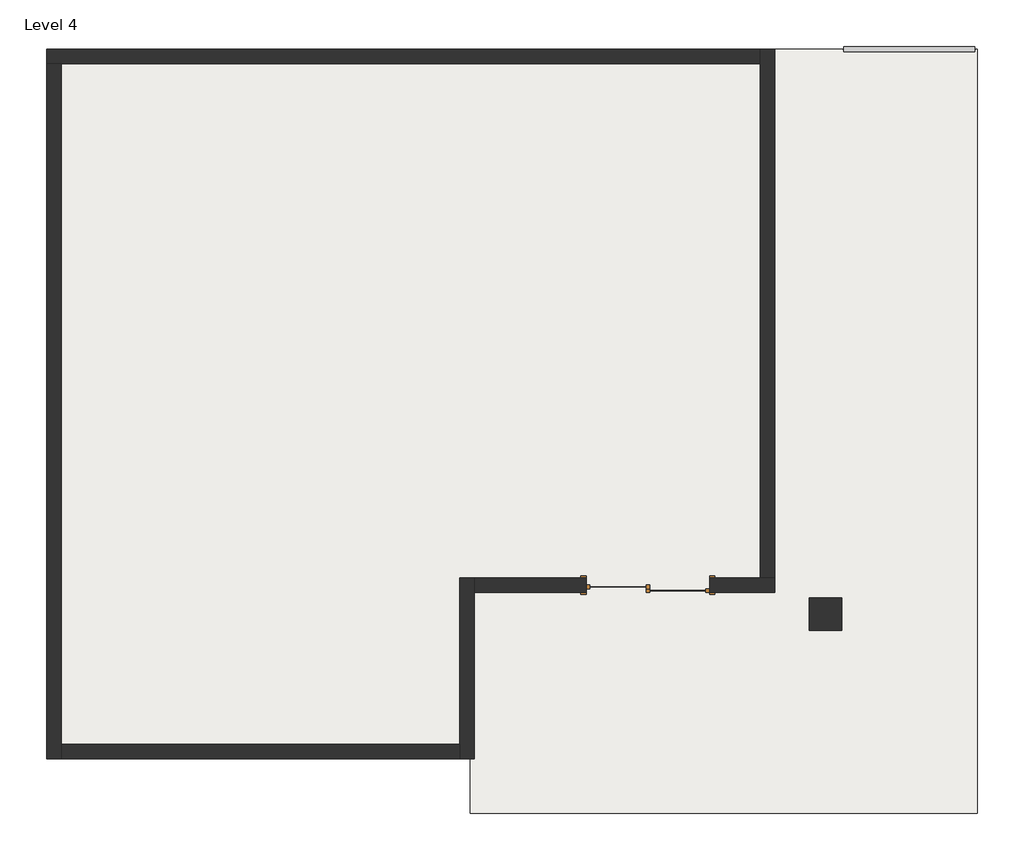
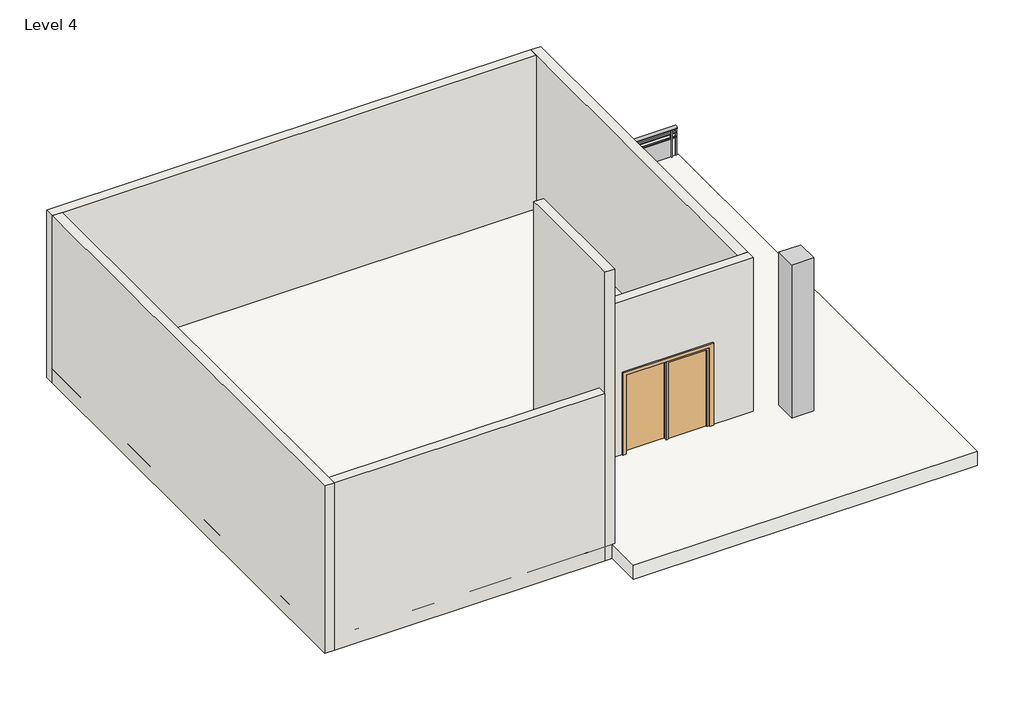
# One storey, incomplete: 6 walls, 1 column, 1 door, 1 railing, 1 roof.
"""IFC4 building model written with IfcOpenShell, lengths in millimetres."""

from ifc_helpers import new_model, si_unit, point, frame, origin, place, context, project, spatial, polyline, ellipse_curve, trimmed, outline, extrude, faceted_brep, transform, mapped, element, save
from ifc_brep_helpers import plane_surface, extruded_surface, advanced_brep
from components import door_076b30e0

model = new_model("IFC4")

# Units and contexts
model_context = context("Model", 3, world=origin())
ifc_project = project(units=[si_unit("LENGTHUNIT", "METRE", prefix="MILLI")], contexts=[model_context])

# Site, building, storey
site = spatial("IfcSite", under=ifc_project)
building = spatial("IfcBuilding", under=site)
storey = spatial("IfcBuildingStorey", under=building, Name="Level 4", Elevation=10972.8)

# Column
placement = place(None, origin())
element("IfcColumn", 1, ObjectType="Rectangular Column : 18\" x 18\"", at=placement, inside=storey, context=model_context, shape_type="SweptSolid", body=[
    extrude(outline(polyline([(198.6628702, 3405.1359817), (198.6628702, 2947.9359817), (-258.5371298, 2947.9359817), (-258.5371298, 3405.1359817), (198.6628702, 3405.1359817)])), frame((0.0, 0.0, 10972.8), z_axis=(0.0, 0.0, 1.0), x_axis=(1.0, 0.0, 0.0)), (0.0, 0.0, 1.0), 3657.6),
])

# Door
door_shape = door_076b30e0(model_context)
element("IfcDoor", 2, ObjectType="Door-Double-Sliding : 68\" x 80\"", at=placement, inside=storey, context=model_context, shape_type="MappedRepresentation", body=[
    mapped(door_shape, transform((-2519.1371298, 3709.9359817, 10972.8), x_axis=(-1.0, 0.0, 0.0), y_axis=(0.0, -1.0, 0.0), z_axis=(0.0, 0.0, 1.0))),
])

# Railing
element("IfcRailing", 3, ObjectType="Glass Panel - Bottom Fill", at=placement, inside=storey, context=model_context, shape_type="SolidModel", body=[
    advanced_brep(
    [(2062.5612535, 11063.2359817, 11887.2), (2062.5612535, 11139.4359817, 11887.2), (224.0628702, 11063.2359817, 11887.2), (224.0628702, 11139.4359817, 11887.2)],
    [
        (0, 1, ellipse_curve(frame((2062.5612535, 11101.3359817, 11887.2), z_axis=(1.0, 0.0, 0.0), x_axis=(0.0, 1.0, 0.0)), 38.1, 28.575)),
        (1, 0, ellipse_curve(frame((2062.5612535, 11101.3359817, 11887.2), z_axis=(1.0, 0.0, 0.0), x_axis=(0.0, 1.0, 0.0)), 38.1, 28.575)),
        (2, 3, ellipse_curve(frame((224.0628702, 11101.3359817, 11887.2), z_axis=(-1.0, 0.0, 0.0), x_axis=(0.0, 1.0, 0.0)), 38.1, 28.575)),
        (3, 2, ellipse_curve(frame((224.0628702, 11101.3359817, 11887.2), z_axis=(-1.0, 0.0, 0.0), x_axis=(0.0, 1.0, 0.0)), 38.1, 28.575)),
        (0, 2),
        (3, 1),
    ],
    [
        plane_surface(frame((2062.5612535, 11101.3359817, 11887.2), z_axis=(1.0, 0.0, 0.0), x_axis=(0.0, -1.0, 0.0))),
        plane_surface(frame((224.0628702, 11101.3359817, 11887.2), z_axis=(-1.0, 0.0, 0.0), x_axis=(0.0, -1.0, 0.0))),
        extruded_surface(trimmed(ellipse_curve(frame((224.0628702, 11101.3359817, 11887.2), z_axis=(1.0, 0.0, 0.0), x_axis=(0.0, 1.0, 0.0)), 38.1, 28.575), [point((224.0628702, 11063.2359817, 11887.2))], [point((224.0628702, 11139.4359817, 11887.2))], True, "CARTESIAN"), (1838.4983833000001, 0.0, 0.0), 1838.4983833000001),
        extruded_surface(trimmed(ellipse_curve(frame((224.0628702, 11101.3359817, 11887.2), z_axis=(1.0, 0.0, 0.0), x_axis=(0.0, 1.0, 0.0)), 38.1, 28.575), [point((224.0628702, 11139.4359817, 11887.2))], [point((224.0628702, 11063.2359817, 11887.2))], True, "CARTESIAN"), (1838.4983833000001, 0.0, 0.0), 1838.4983833000001),
    ],
    [
        (0, [[1, 2]]),
        (1, [[3, 4]]),
        (2, [[-1, 5, -4, 6]]),
        (3, [[-2, -6, -3, -5]]),
    ],
),
    extrude(outline(polyline([(2062.5612535, 11114.0359817), (2062.5612535, 11088.6359817), (224.0628702, 11088.6359817), (224.0628702, 11114.0359817), (2062.5612535, 11114.0359817)])), frame((0.0, 0.0, 11772.9), z_axis=(0.0, 0.0, 1.0), x_axis=(1.0, 0.0, 0.0)), (0.0, 0.0, 1.0), 25.4),
    extrude(outline(polyline([(2062.5612535, 11114.0359817), (2062.5612535, 11088.6359817), (224.0628702, 11088.6359817), (224.0628702, 11114.0359817), (2062.5612535, 11114.0359817)])), frame((0.0, 0.0, 11671.3), z_axis=(0.0, 0.0, 1.0), x_axis=(1.0, 0.0, 0.0)), (0.0, 0.0, 1.0), 25.4),
    extrude(outline(polyline([(336.8620618, 11126.7359817), (336.8620618, 11075.9359817), (324.1620618, 11075.9359817), (324.1620618, 11126.7359817), (336.8620618, 11126.7359817)])), frame((0.0, 0.0, 10972.8), z_axis=(0.0, 0.0, 1.0), x_axis=(1.0, 0.0, 0.0)), (0.0, 0.0, 1.0), 885.6788223),
    extrude(outline(polyline([(1143.3120618, 11094.8008247), (330.5120618, 11094.8008247), (330.5120618, 11101.1508247), (1143.3120618, 11101.1508247), (1143.3120618, 11094.8008247)])), frame((0.0, 0.0, 11074.4), z_axis=(0.0, 0.0, 1.0), x_axis=(1.0, 0.0, 0.0)), (0.0, 0.0, 1.0), 596.9),
    extrude(outline(polyline([(1149.6620618, 11126.7359817), (1149.6620618, 11075.9359817), (1136.9620618, 11075.9359817), (1136.9620618, 11126.7359817), (1149.6620618, 11126.7359817)])), frame((0.0, 0.0, 10972.8), z_axis=(0.0, 0.0, 1.0), x_axis=(1.0, 0.0, 0.0)), (0.0, 0.0, 1.0), 885.6788223),
    extrude(outline(polyline([(1956.1120618, 11094.8008247), (1143.3120618, 11094.8008247), (1143.3120618, 11101.1508247), (1956.1120618, 11101.1508247), (1956.1120618, 11094.8008247)])), frame((0.0, 0.0, 11074.4), z_axis=(0.0, 0.0, 1.0), x_axis=(1.0, 0.0, 0.0)), (0.0, 0.0, 1.0), 596.9),
    extrude(outline(polyline([(1962.4620618, 11126.7359817), (1962.4620618, 11075.9359817), (1949.7620618, 11075.9359817), (1949.7620618, 11126.7359817), (1962.4620618, 11126.7359817)])), frame((0.0, 0.0, 10972.8), z_axis=(0.0, 0.0, 1.0), x_axis=(1.0, 0.0, 0.0)), (0.0, 0.0, 1.0), 885.6788223),
    extrude(outline(polyline([(236.7628702, 11110.8609817), (236.7628702, 11091.8109817), (217.7128702, 11091.8109817), (217.7128702, 11110.8609817), (236.7628702, 11110.8609817)])), frame((0.0, 0.0, 10972.8), z_axis=(0.0, 0.0, 1.0), x_axis=(1.0, 0.0, 0.0)), (0.0, 0.0, 1.0), 885.6788223),
    extrude(outline(polyline([(2068.9112535, 11110.8609817), (2068.9112535, 11091.8109817), (2049.8612535, 11091.8109817), (2049.8612535, 11110.8609817), (2068.9112535, 11110.8609817)])), frame((0.0, 0.0, 10972.8), z_axis=(0.0, 0.0, 1.0), x_axis=(1.0, 0.0, 0.0)), (0.0, 0.0, 1.0), 885.6788223),
])

# Roof
element("IfcRoof", 4, ObjectType="Generic - 12\"", at=placement, inside=storey, context=model_context, shape_type="SweptSolid", body=[
    extrude(outline(polyline([(-10951.9371298, 11101.3359817), (2101.2415497, 11101.3359817), (2101.2415497, 1144.5359817), (2101.2415497, 382.5359817), (-5008.3371298, 382.5359817), (-5008.3371298, 1144.5359817), (-10951.9371298, 1144.5359817), (-10951.9371298, 11101.3359817)])), frame((0.0, 0.0, 10972.8), z_axis=(0.0, 0.0, 1.0), x_axis=(1.0, 0.0, 0.0)), (0.0, 0.0, 1.0), 304.8),
])

# Walls
element("IfcWall", 5, ObjectType="Generic - 8\"", at=placement, inside=storey, context=model_context, shape_type="Brep", body=[
    faceted_brep([(-10951.9371298, 10898.1359817, 10972.8), (-10748.7371298, 10898.1359817, 10972.8), (-944.3371298, 10898.1359817, 10972.8), (-944.3371298, 10898.1359817, 14630.4), (-10748.7371298, 10898.1359817, 14630.4), (-10951.9371298, 10898.1359817, 14630.4), (-10951.9371298, 11101.3359817, 10972.8), (-10951.9371298, 11101.3359817, 14630.4), (-944.3371298, 11101.3359817, 14630.4), (-944.3371298, 11101.3359817, 10972.8)], [[[0, 1, 2, 3, 4, 5]], [[6, 7, 8, 9]], [[2, 1, 0, 6, 9]], [[5, 4, 3, 8, 7]], [[0, 5, 7, 6]], [[3, 2, 9, 8]]]),
])
element("IfcWall", 6, ObjectType="Generic - 8\"", at=placement, inside=storey, context=model_context, shape_type="Brep", body=[
    faceted_brep([(-10748.7371298, 1144.5359817, 10972.8), (-10748.7371298, 1347.7359817, 10972.8), (-10748.7371298, 10898.1359817, 10972.8), (-10748.7371298, 10898.1359817, 14630.4), (-10748.7371298, 1347.7359817, 14630.4), (-10748.7371298, 1144.5359817, 14630.4), (-10951.9371298, 1144.5359817, 10972.8), (-10951.9371298, 1144.5359817, 14630.4), (-10951.9371298, 10898.1359817, 14630.4), (-10951.9371298, 10898.1359817, 10972.8)], [[[0, 1, 2, 3, 4, 5]], [[6, 7, 8, 9]], [[2, 1, 0, 6, 9]], [[5, 4, 3, 8, 7]], [[0, 5, 7, 6]], [[3, 2, 9, 8]]]),
])
element("IfcWall", 7, ObjectType="Generic - 8\"", at=placement, inside=storey, context=model_context, shape_type="SweptSolid", body=[
    extrude(outline(polyline([(-10748.7371298, 1347.7359817), (-5160.7371298, 1347.7359817), (-5160.7371298, 1144.5359817), (-10748.7371298, 1144.5359817), (-10748.7371298, 1347.7359817)])), frame((0.0, 0.0, 10972.8), z_axis=(0.0, 0.0, 1.0), x_axis=(1.0, 0.0, 0.0)), (0.0, 0.0, 1.0), 3657.6),
])
element("IfcWall", 8, ObjectType="Generic - 8\"", at=placement, inside=storey, context=model_context, shape_type="Brep", body=[
    faceted_brep([(-944.3371298, 11101.3359817, 10972.8), (-944.3371298, 10898.1359817, 10972.8), (-944.3371298, 3684.5359817, 10972.8), (-944.3371298, 3684.5359817, 14630.4), (-944.3371298, 10898.1359817, 14630.4), (-944.3371298, 11101.3359817, 14630.4), (-741.1371298, 11101.3359817, 10972.8), (-741.1371298, 11101.3359817, 14630.4), (-741.1371298, 3684.5359817, 14630.4), (-741.1371298, 3684.5359817, 10972.8)], [[[0, 1, 2, 3, 4, 5]], [[6, 7, 8, 9]], [[2, 1, 0, 6, 9]], [[5, 4, 3, 8, 7]], [[0, 5, 7, 6]], [[3, 2, 9, 8]]]),
])
element("IfcWall", 9, ObjectType="Generic - 8\"", at=placement, inside=storey, context=model_context, shape_type="Brep", body=[
    faceted_brep([(-4957.5371298, 1144.5359817, 10972.8), (-4957.5371298, 3481.3359817, 10972.8), (-4957.5371298, 3684.5359817, 10972.8), (-4957.5371298, 3684.5359817, 14630.4), (-4957.5371298, 3684.5359817, 17282.1203125), (-4957.5371298, 1144.5359817, 17282.1203125), (-5160.7371298, 1144.5359817, 10972.8), (-5160.7371298, 1144.5359817, 14630.4), (-5160.7371298, 1144.5359817, 17282.1203125), (-5160.7371298, 3481.3359817, 17282.1203125), (-5160.7371298, 3684.5359817, 17282.1203125), (-5160.7371298, 3684.5359817, 14630.4), (-5160.7371298, 3684.5359817, 10972.8), (-5160.7371298, 1347.7359817, 10972.8)], [[[0, 1, 2, 3, 4, 5]], [[6, 7, 8, 9, 10, 11, 12, 13]], [[2, 1, 0, 6, 13, 12]], [[5, 4, 10, 9, 8]], [[0, 5, 8, 7, 6]], [[2, 12, 11, 10, 4, 3]]]),
])
element("IfcWall", 10, ObjectType="Generic - 8\"", at=placement, inside=storey, context=model_context, shape_type="Brep", body=[
    faceted_brep([(-4957.5371298, 3481.3359817, 10972.8), (-3382.7371298, 3481.3359817, 10972.8), (-3382.7371298, 3481.3359817, 13004.8), (-1655.5371298, 3481.3359817, 13004.8), (-1655.5371298, 3481.3359817, 10972.8), (-741.1371298, 3481.3359817, 10972.8), (-741.1371298, 3481.3359817, 14630.4), (-4957.5371298, 3481.3359817, 14630.4), (-3382.7371298, 3684.5359817, 13004.8), (-3382.7371298, 3684.5359817, 10972.8), (-4957.5371298, 3684.5359817, 10972.8), (-4957.5371298, 3684.5359817, 14630.4), (-944.3371298, 3684.5359817, 14630.4), (-741.1371298, 3684.5359817, 14630.4), (-741.1371298, 3684.5359817, 10972.8), (-944.3371298, 3684.5359817, 10972.8), (-1655.5371298, 3684.5359817, 10972.8), (-1655.5371298, 3684.5359817, 13004.8)], [[[0, 1, 2, 3, 4, 5, 6, 7]], [[8, 9, 10, 11, 12, 13, 14, 15, 16, 17]], [[10, 9, 1, 0]], [[16, 15, 14, 5, 4]], [[7, 6, 13, 12, 11]], [[0, 7, 11, 10]], [[6, 5, 14, 13]], [[4, 3, 17, 16]], [[2, 1, 9, 8]], [[3, 2, 8, 17]]]),
])

save(model, "model.ifc")

# Revit data of these elements
# Type "Rectangular Column : 18\" x 18\""
#   Assembly Code = "B1010200"
#   Depth = 1' - 6"
#   Offset Base = 0' - 0"
#   Offset Top = 0' - 0"
#   Width = 1' - 6"
#   Material = none
# Type "Door-Double-Sliding : 68\" x 80\""
#   Type Mark = "9"
#   Construction Type Id = "opn-d45"
#   Assembly Code = "C1020"
#   Analytic Construction = "Wood frame, double glass door "
#   Thickness = 0' - 2"
#   Thermal Resistance (R) = 1.8150 (h·ft²·°F)/BTU
#   Heat Transfer Coefficient (U) = 0.5510 BTU/(h·ft²·°F)
#   Height = 6' - 8"
#   Rail Width = 0' - 2"
#   Stiles = 0' - 2"
#   Trim Projection Ext = 0' - 1"
#   Trim Projection Int = 0' - 1"
#   Trim Width = 0' - 3"
#   Width = 5' - 8"
#   Define Thermal Properties by = 1
#   Glazing = Glass
#   Panel Material = Wood - Birch - Solid Stained Light Low Gloss
#   Trim Material = Paint - Sienna
#   Visual Light Transmittance = 0
#   Solar Heat Gain Coefficient = 0
#   Function = (empty or 0)
#   Wall Closure = (empty or 0)
# Type "Glass Panel - Bottom Fill"
#   Assembly Code = "C2010400"
#   built-in parameter 1008612 = 0.0416667 (stored number, unit not read)
#   built-in parameter 1008611 = 0.0416667 (stored number, unit not read)
#   built-in parameter 1008609 = 0.333333 (stored number, unit not read)
#   built-in parameter 1008604 = 0.166667 (stored number, unit not read)
#   built-in parameter 1008603 = 0.166667 (stored number, unit not read)
#   Railing Height = 3' - 0"
#   built-in parameter 1008630 = 2
#   built-in parameter 1008610 = 2
#   built-in parameter 1008618 = Baluster - Square : 3/4"
# Type "Generic - 12\""
#   Assembly Code = "B1020"
#   Layers, outside or top first: 1' - 0" no material (function 1)
# Type "Generic - 8\""
#   Assembly Code = "B2010"
#   Layers, outside or top first: 0' - 8" no material (function 1)
# Element 1 (IfcColumn, "Rectangular Column : 18\" x 18\"")
#   Phase Created = New Construction
# Element 2 (IfcDoor, "Door-Double-Sliding : 68\" x 80\"")
#   Phase Created = New Construction
#   Materials on its faces: "Paint - Sienna", "Wood - Birch - Solid Stained Light Low Gloss", "Glass"
# Element 3 (IfcRailing, "Glass Panel - Bottom Fill")
#   Phase Created = New Construction
#   Materials on its faces: "Glass"
# Element 4 (IfcRoof, "Generic - 12\"")
#   built-in parameter 1001705 = 37 (stored number, unit not read)
#   built-in parameter 1001710 = 33615
#   Phase Created = New Construction
#   Materials on its faces: "Default Roof"
# Elements 5, 6, 7, 8, 10 (IfcWall, "Generic - 8\"")
#   Top Offset = 0' - 0"
#   Base Offset = 0' - 0"
#   Unconnected Height = 12' - 0"
#   wall height = 12' - 0"
#   Phase Created = New Construction
#   Base Constraint = Level 4
#   Materials on its faces: "Default Wall"
# Element 9 (IfcWall, "Generic - 8\"")
#   Top Offset = 0' - 0"
#   Base Offset = 0' - 0"
#   Unconnected Height = 20' - 8 51/128"
#   wall height = 20' - 8 51/128"
#   Phase Created = New Construction
#   Base Constraint = Level 4
#   Materials on its faces: "Default Wall"
# Materials
#   "Glass": class "Glass", colour RGB 0 128 192, transparency 0.75, Description = "Soda Lime Glass", Cost = 0
#   "Wood - Birch - Solid Stained Light Low Gloss": class "Wood", colour RGB 210 159 95, transparency 0, Cost = 0
#   "Paint - Sienna": colour RGB 118 70 51, transparency 0, Cost = 0
#   "Default Roof": colour RGB 88 101 114, transparency 0
#   "Default Wall": colour RGB 128 128 128, transparency 0
